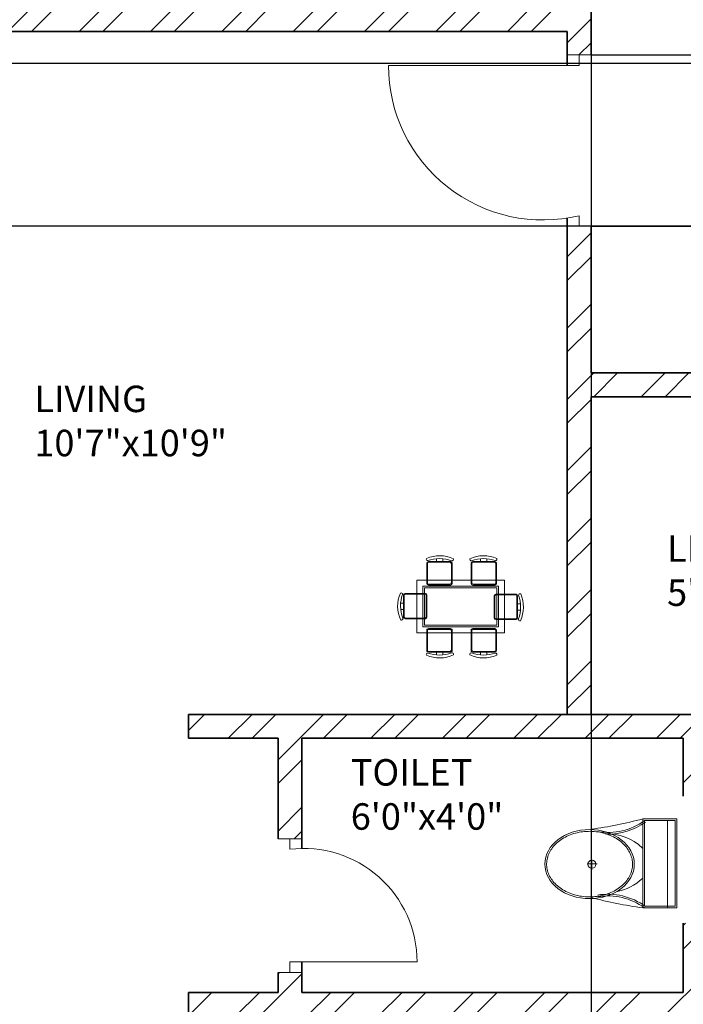
# Model space of a CAD drawing. Units: inches. Extents: x 1570 to 2186, y 1575 to 2421.
# Tile 3 of 10: x 1708 to 1833, y 1859 to 2045. Entities that reach past the tile are written whole.
import ezdxf

# ---------------------------------------------------------------- set-up
doc = ezdxf.new("R2010")
doc.units = ezdxf.units.IN
for name, color, linetype, lineweight in [('A-ANNO-DIMS', 2, 'Continuous', 18), ('A-AREA-IDEN', 7, 'Continuous', 18), ('A-DOOR', 201, 'Continuous', 18), ('A-FLOR-FIXT', 9, 'Continuous', 18), ('A-FURN', 8, 'Continuous', 13), ('A-WALL', 7, 'Continuous', 35), ('A-WALL-PATT', 252, 'Continuous', 13)]:
    doc.layers.add(name, color=color, linetype=linetype, lineweight=lineweight)
doc.styles.get("Standard").update_dxf_attribs({"font": 'arial.ttf'})
doc.dimstyles.get("Standard").update_dxf_attribs({"dimtxt": 0.18, "dimasz": 0.18, "dimexe": 0.18, "dimexo": 0.0625, "dimgap": 0.09, "dimtad": 0, "dimtih": 1, "dimtoh": 1, "dimdec": 4, "dimzin": 0, "dimdsep": 46, "dimtxsty": 'Standard', "dimcen": 0.09, "dimadec": 0, "dimazin": 0, "dimtfac": 1, "dimtdec": 4, "dimtofl": 0, "dimtmove": 0, "dimatfit": 3, "dimfxl": 1, "dimtolj": 1, "dimtzin": 0, "dimarcsym": 0})

# ---------------------------------------------------------------- blocks, each defined once
blk = doc.blocks.new('A$C31115884')
for p, q in [((257.5, 466.4), (257.5, 523.2)), ((283.1, 497.7), (223.4, 497.7)), ((0, 200), (0, 0)), ((520, 200), (0, 200)), ((10, 190), (10, 10)), ((510, 190), (10, 190)), ((510, 10), (510, 190)), ((520, 0), (520, 200)), ((510, 54.5), (0, 54.5)), ((10, 10), (510, 10)), ((0, 0), (520, 0))]:
    blk.add_line(p, q)
blk.add_circle((255.6, 496.4), 23.6)
for centre, radius, start, end in [((2777.7, -204.6), 2807, 165.4549, 171.71327), ((-294.5, 403.3), 364.7, 324.20913, 9.34987), ((-294.5, 403.3), 374.7, 324.20913, 9.34987), ((805.8, 403.3), 364.7, 170.65013, 215.79087), ((3237, 905), 2807, 188.28673, 194.5451), ((139.5, 406.2), 293.5, 315.84364, 2.65635), ((805.8, 403.3), 374.7, 179.20365, 215.79087), ((383.6, 406.2), 293.5, 190.27735, 224.15636)]:
    blk.add_arc(centre, radius, start, end)
blk.add_ellipse((256.2, 509.9), major_axis=(0, -260.7), ratio=0.772727)
blk.add_open_spline([(256.2, 259.2), (263.1, 259.2), (270, 259.7), (287.8, 262.3), (298.7, 265.1), (319.9, 273.1), (330.2, 278.4), (350.1, 291.1), (359.7, 298.7), (377.7, 315.9), (386.2, 325.5), (401.7, 346.6), (408.8, 358.1), (421.3, 382.5), (426.8, 395.5), (435.9, 422.4), (439.5, 436.4), (444.8, 465.1), (446.5, 479.7), (447.9, 509.2), (447.6, 524), (445, 553.3), (442.7, 567.8), (436.3, 596), (432.1, 609.7), (421.9, 636), (416, 648.6), (402.5, 672.1), (395, 683), (378.6, 703), (369.8, 712.1), (351.1, 728), (341.3, 734.8), (320.9, 746.2), (310.4, 750.7), (288.9, 757.3), (278, 759.4), (256, 761), (245, 760.6), (223.1, 757.2), (212.3, 754.3), (191.1, 746.1), (180.8, 740.7), (160.9, 727.8), (151.4, 720.1), (133.5, 702.7), (125.1, 693), (109.6, 671.7), (102.6, 660.2), (90.2, 635.7), (84.9, 622.7), (76, 595.6), (72.4, 581.6), (67.2, 552.9), (65.6, 538.2), (64.4, 508.8), (64.8, 494), (67.5, 464.7), (69.9, 450.2), (76.6, 422), (80.8, 408.3), (91.1, 382.2), (97.2, 369.7), (110.8, 346.3), (118.4, 335.4), (134.8, 315.6), (143.7, 306.7), (162.4, 290.9), (172.3, 284.2), (192.8, 273), (203.3, 268.6), (224.8, 262.2), (235.8, 260.2), (249.9, 259.3), (253, 259.2), (256.2, 259.2)], degree=3, knots=[0, 0, 0, 0, 0.110105, 0.110105, 0.285049, 0.285049, 0.459994, 0.459994, 0.634938, 0.634938, 0.809882, 0.809882, 0.984827, 0.984827, 1.159771, 1.159771, 1.334715, 1.334715, 1.50966, 1.50966, 1.684604, 1.684604, 1.859549, 1.859549, 2.034493, 2.034493, 2.209437, 2.209437, 2.384382, 2.384382, 2.559326, 2.559326, 2.73427, 2.73427, 2.909215, 2.909215, 3.084159, 3.084159, 3.259103, 3.259103, 3.434048, 3.434048, 3.608992, 3.608992, 3.783936, 3.783936, 3.958881, 3.958881, 4.133825, 4.133825, 4.30877, 4.30877, 4.483714, 4.483714, 4.658658, 4.658658, 4.833603, 4.833603, 5.008547, 5.008547, 5.183491, 5.183491, 5.358436, 5.358436, 5.53338, 5.53338, 5.708324, 5.708324, 5.883269, 5.883269, 6.058213, 6.058213, 6.233158, 6.233158, 6.283185, 6.283185, 6.283185, 6.283185])
blk = doc.blocks.new('TABLE-DINING')
for points in [[(0, 9.93), (16.54, 9.93), (16.54, 0), (0, 0)], [(0, 9.93), (16.54, 9.93), (16.54, 0), (0, 0)], [(1.1, 8.82), (15.44, 8.82), (15.44, 1.1), (1.1, 1.1)], [(1.1, 8.82), (15.44, 8.82), (15.44, 1.1), (1.1, 1.1)], [(1.43, 8.49), (15.11, 8.49), (15.11, 1.43), (1.43, 1.43)], [(1.43, 8.49), (15.11, 8.49), (15.11, 1.43), (1.43, 1.43)]]:
    blk.add_lwpolyline(points, close=True)
blk = doc.blocks.new('DINING-CHAIR-LH')
for points in [[(4.59, 1.1), (0.4, 1.1, -0.414214), (0.11, 1.39), (0.11, 5.24, -0.414214), (0.4, 5.53), (4.59, 5.53, -0.414214), (4.88, 5.24), (4.88, 1.39, -0.414214), (4.59, 1.1)], [(4.59, 1.1), (0.4, 1.1, -0.414214), (0.11, 1.39), (0.11, 5.24, -0.414214), (0.4, 5.53), (4.59, 5.53, -0.414214), (4.88, 5.24), (4.88, 1.39, -0.414214), (4.59, 1.1)], [(4.78, 0.96, -0.578392), (5.12, 0.58, -0.214524), (0.03, 0.51, -0.552014), (0.27, 0.92, 0.175809), (4.78, 0.96)], [(4.78, 0.96, -0.578392), (5.12, 0.58, -0.214524), (0.03, 0.51, -0.552014), (0.27, 0.92, 0.175809), (4.78, 0.96)], [(3.12, 1.1), (3.12, 0.57, 0.064759)], [(3.12, 1.1), (3.12, 0.57, 0.064759)]]:
    blk.add_lwpolyline(points, format="xyb")
blk.add_lwpolyline([(0.4, 1.23), (4.45, 1.23, 0.414214), (4.75, 1.53), (4.75, 5.11, 0.414214), (4.45, 5.4), (0.4, 5.4, 0.512069), (0.24, 5.11), (0.24, 1.53, 0.512069)], format="xyb", close=True)
blk.add_lwpolyline([(0.4, 1.23), (4.45, 1.23, 0.414214), (4.75, 1.53), (4.75, 5.11, 0.414214), (4.45, 5.4), (0.4, 5.4, 0.512069), (0.24, 5.11), (0.24, 1.53, 0.512069)], format="xyb", close=True)
blk.add_lwpolyline([(1.95, 0.56), (1.95, 1.1)])
blk.add_lwpolyline([(1.95, 0.56), (1.95, 1.1)])
blk = doc.blocks.new('DINING-CHAIR-RH')
for points in [[(4.73, 1.1, 0.414214), (5.02, 1.39), (5.02, 5.24, 0.414214), (4.73, 5.53), (0.55, 5.53, 0.414214), (0.25, 5.24), (0.25, 1.39, 0.414214), (0.55, 1.1), (4.73, 1.1)], [(4.73, 1.1, 0.414214), (5.02, 1.39), (5.02, 5.24, 0.414214), (4.73, 5.53), (0.55, 5.53, 0.414214), (0.25, 5.24), (0.25, 1.39, 0.414214), (0.55, 1.1), (4.73, 1.1)], [(4.86, 0.92, -0.175809), (0.35, 0.96, 0.578392), (0.01, 0.58, 0.214524), (5.1, 0.51, 0.552014), (4.86, 0.92, -0.065079)], [(4.86, 0.92, -0.175809), (0.35, 0.96, 0.578392), (0.01, 0.58, 0.214524), (5.1, 0.51, 0.552014), (4.86, 0.92, -0.065079)], [(2.02, 1.1), (2.02, 0.57, -0.064759)], [(2.02, 1.1), (2.02, 0.57, -0.064759)]]:
    blk.add_lwpolyline(points, format="xyb")
blk.add_lwpolyline([(4.73, 1.23), (0.68, 1.23, -0.414214), (0.39, 1.53), (0.39, 5.11, -0.414214), (0.68, 5.4), (4.73, 5.4, -0.512069), (4.89, 5.11), (4.89, 1.53, -0.512069)], format="xyb", close=True)
blk.add_lwpolyline([(4.73, 1.23), (0.68, 1.23, -0.414214), (0.39, 1.53), (0.39, 5.11, -0.414214), (0.68, 5.4), (4.73, 5.4, -0.512069), (4.89, 5.11), (4.89, 1.53, -0.512069)], format="xyb", close=True)
blk.add_lwpolyline([(3.19, 0.56), (3.19, 1.1)])
blk.add_lwpolyline([(3.19, 0.56), (3.19, 1.1)])
blk = doc.blocks.new('*D39')
at = {"layer": 'A-ANNO-DIMS', "color": 0, "lineweight": -2, "transparency": 16777216}
for p, q in [((1816.09, 2097.8), (1816.09, 1616.73)), ((1913.59, 2097.8), (1913.59, 1616.73)), ((1816.27, 1616.91), (1864.51, 1616.91)), ((1913.41, 1616.91), (1865.16, 1616.91))]:
    blk.add_line(p, q, dxfattribs=at)
at = {"layer": 'A-ANNO-DIMS', "color": 0, "transparency": 16777216}
for points in [[(1816.27, 1616.94), (1816.27, 1616.88), (1816.09, 1616.91)], [(1913.41, 1616.94), (1913.41, 1616.88), (1913.59, 1616.91)]]:
    blk.add_solid(points, dxfattribs=at)
at = {"layer": 'Defpoints', "color": 0, "transparency": 16777216}
for p in [(1816.09, 2097.86), (1913.59, 2097.86), (1913.59, 1616.91)]:
    blk.add_point(p, dxfattribs=at)
at = {"layer": 'A-ANNO-DIMS', "color": 0, "transparency": 16777216, "insert": (1864.84, 1616.91), "char_height": 0.18, "attachment_point": 5}
blk.add_mtext('\\A1;97.5', dxfattribs=at)
blk = doc.blocks.new('*D41')
at = {"layer": 'A-ANNO-DIMS', "color": 0, "lineweight": -2, "transparency": 16777216}
for p, q in [((1816.15, 2038.3), (2126.57, 2038.3)), ((2126.39, 2038.12), (2126.39, 2022.3)), ((2126.39, 2006.11), (2126.39, 2021.93)), ((1816.15, 2005.93), (2126.57, 2005.93))]:
    blk.add_line(p, q, dxfattribs=at)
at = {"layer": 'A-ANNO-DIMS', "color": 0, "transparency": 16777216}
for points in [[(2126.36, 2038.12), (2126.42, 2038.12), (2126.39, 2038.3)], [(2126.36, 2006.11), (2126.42, 2006.11), (2126.39, 2005.93)]]:
    blk.add_solid(points, dxfattribs=at)
at = {"layer": 'Defpoints', "color": 0, "transparency": 16777216}
for p in [(1816.09, 2038.3), (2126.39, 2038.3), (1816.09, 2005.93)]:
    blk.add_point(p, dxfattribs=at)
at = {"layer": 'A-ANNO-DIMS', "color": 0, "transparency": 16777216, "insert": (2126.39, 2022.12), "char_height": 0.18, "attachment_point": 5}
blk.add_mtext('\\A1;32.365', dxfattribs=at)
blk = doc.blocks.new('*D43')
at = {"layer": 'A-ANNO-DIMS', "color": 0, "lineweight": -2, "transparency": 16777216}
for p, q in [((1913.53, 2036.69), (1603.11, 2036.69)), ((1603.29, 2036.51), (1603.29, 2021.49)), ((1603.29, 2006.11), (1603.29, 2021.13)), ((1913.53, 2005.93), (1603.11, 2005.93))]:
    blk.add_line(p, q, dxfattribs=at)
at = {"layer": 'A-ANNO-DIMS', "color": 0, "transparency": 16777216}
for points in [[(1603.26, 2036.51), (1603.32, 2036.51), (1603.29, 2036.69)], [(1603.26, 2006.11), (1603.32, 2006.11), (1603.29, 2005.93)]]:
    blk.add_solid(points, dxfattribs=at)
at = {"layer": 'Defpoints', "color": 0, "transparency": 16777216}
for p in [(1603.29, 2036.69), (1913.59, 2036.69), (1913.59, 2005.93)]:
    blk.add_point(p, dxfattribs=at)
at = {"layer": 'A-ANNO-DIMS', "color": 0, "transparency": 16777216, "insert": (1603.29, 2021.31), "char_height": 0.18, "attachment_point": 5}
blk.add_mtext('\\A1;30.753', dxfattribs=at)

msp = doc.modelspace()

# ---------------------------------------------------------------- hatches: boundary and pattern name
at = {"layer": 'A-WALL-PATT'}
h = msp.add_hatch(dxfattribs=at)
h.set_pattern_fill('ANSI32', color=256)
h.paths.add_polyline_path([(1762.0975, 2362.1492), (1757.5975, 2362.1492), (1757.5975, 2357.6492), (1709.1163, 2357.6492), (1709.1163, 2362.1492), (1704.6163, 2362.1492), (1704.6163, 2353.1492), (1740.0886, 2353.1492), (1740.0886, 2261.8115), (1744.5886, 2261.8115), (1744.5886, 2353.1492), (1762.0975, 2353.1492)])
h.paths.add_polyline_path([(1890.2592, 2362.1492), (1885.7592, 2362.1492), (1826.5975, 2362.1492), (1822.0975, 2362.1492), (1822.0975, 2353.1492), (1862.5886, 2353.1492), (1862.5886, 2227.1492), (1744.5886, 2227.1492), (1744.5886, 2229.5389), (1742.3386, 2229.5389), (1740.0886, 2229.5389), (1740.0886, 2222.6492), (1744.5886, 2222.6492), (1756.186, 2222.6492), (1756.186, 2216.3571), (1760.686, 2216.3571), (1760.686, 2222.6492), (1832.686, 2222.6492), (1832.686, 2212.5994), (1837.186, 2212.5994), (1837.186, 2222.6492), (1893.186, 2222.6492), (1893.186, 2212.5994), (1897.686, 2212.5994), (1897.686, 2222.6492), (1989.5886, 2222.6492), (1989.5886, 2227.1492), (1989.5886, 2232.6585), (1987.3386, 2232.6585), (1985.0886, 2232.6585), (1985.0886, 2227.1492), (1867.0886, 2227.1492), (1867.0886, 2353.1492), (1890.2592, 2353.1492)])
h.paths.add_polyline_path([(1644.0886, 2353.1492), (1668.6163, 2353.1492), (1668.6163, 2362.1492), (1664.1163, 2362.1492), (1664.1163, 2358.9932), (1664.1163, 2357.6492), (1639.5886, 2357.6492), (1639.5886, 2213.8746), (1644.0886, 2213.8746), (1644.0886, 2222.6492), (1692.0886, 2222.6492), (1692.0886, 2215.9343), (1696.5886, 2215.9343), (1696.5886, 2222.6492), (1696.5886, 2227.1492), (1644.0886, 2227.1492)])
h.paths.add_polyline_path([(2013.0435, 2362.1492), (2008.5435, 2362.1492), (2008.5435, 2357.6492), (1954.7592, 2357.6492), (1954.7592, 2362.1492), (1950.2592, 2362.1492), (1950.2592, 2353.1492), (1985.0886, 2353.1492), (1985.0886, 2260.8534), (1989.5886, 2260.8534), (1989.5886, 2353.1492), (2013.0435, 2353.1492)])
h.paths.add_polyline_path([(2090.0886, 2357.6492), (2053.5435, 2357.6492), (2053.5435, 2362.1492), (2049.0435, 2362.1492), (2049.0435, 2353.1492), (2085.5886, 2353.1492), (2085.5886, 2227.1492), (2033.0886, 2227.1492), (2033.0886, 2222.6492), (2033.0886, 2214.4464), (2037.5886, 2214.4464), (2037.5886, 2222.6492), (2085.5886, 2222.6492), (2085.5886, 2212.4409), (2090.0886, 2212.4409)])
h.paths.add_polyline_path([(2090.0886, 2188.4409), (2087.8386, 2188.4409), (2085.5886, 2188.4409), (2085.5886, 2180.6492), (2037.5886, 2180.6492), (2037.5886, 2196.7956), (2033.0886, 2196.7956), (2033.0886, 2176.1492), (2037.5886, 2176.1492), (2045.0886, 2176.1492), (2045.0886, 2169.8988), (2049.5886, 2169.8988), (2049.5886, 2176.1492), (2085.5886, 2176.1492), (2085.5886, 2167.785), (2090.0886, 2167.785)])
h.paths.add_polyline_path([(2049.5886, 2147.4502), (2047.3386, 2147.4502), (2045.0886, 2147.4502), (2045.0886, 2124.4703), (2049.5886, 2124.4703)])
h.paths.add_polyline_path([(2090.0886, 2047.1492), (2049.5886, 2047.1492), (2049.5886, 2064.4703), (2045.0886, 2064.4703), (2045.0886, 2047.1492), (1918.0886, 2047.1492), (1918.0886, 2051.2061), (1913.5886, 2051.2061), (1913.5886, 2047.1492), (1913.5886, 2036.6872), (1918.0886, 2036.6872), (1918.0886, 2042.7492), (2045.0886, 2042.7492), (2045.0886, 2027.0686), (2049.5886, 2027.0686), (2049.5886, 2042.7492), (2090.0886, 2042.7492)])
h.paths.add_polyline_path([(1918.0886, 2005.9338), (1915.8386, 2005.9338), (1913.5886, 2005.9338), (1913.5886, 1913.7492), (1918.0886, 1913.7492)])
h.paths.add_polyline_path([(2090.0886, 1913.7492), (2049.5886, 1913.7492), (2045.0886, 1913.7492), (2033.0886, 1913.7492), (2033.0886, 1909.2492), (2033.0886, 1900.9803), (2037.5886, 1900.9803), (2037.5886, 1909.2492), (2085.5886, 1909.2492), (2085.5886, 1861.2492), (2037.5886, 1861.2492), (2037.5886, 1880.0859), (2033.0886, 1880.0859), (2033.0886, 1856.7492), (2085.5886, 1856.7492), (2085.5886, 1730.7492), (2054.2483, 1730.7492), (2054.2483, 1721.7492), (2058.7483, 1721.7492), (2058.7483, 1726.2492), (2090.0886, 1726.2492)])
h.paths.add_polyline_path([(2049.5886, 1967.0686), (2045.0886, 1967.0686), (2045.0886, 1913.7492), (2049.5886, 1913.7492)])
h.paths.add_polyline_path([(1989.5886, 1824.1695), (1987.3386, 1824.1695), (1985.0886, 1824.1695), (1985.0886, 1730.7492), (1989.5886, 1730.7492)])
h.paths.add_polyline_path([(1989.5886, 1861.2492), (1974.9963, 1861.2492), (1974.9963, 1865.9306), (1972.7463, 1865.9306), (1970.4963, 1865.9306), (1970.4963, 1861.2492), (1898.4963, 1861.2492), (1898.4963, 1874.2999), (1893.9963, 1874.2999), (1893.9963, 1861.2492), (1890.5886, 1861.2492), (1837.9963, 1861.2492), (1837.9963, 1874.3159), (1833.4963, 1874.3159), (1833.4963, 1861.2492), (1761.4963, 1861.2492), (1761.4963, 1865.0209), (1759.2463, 1865.0209), (1756.9963, 1865.0209), (1756.9963, 1861.2492), (1740.0886, 1861.2492), (1740.0886, 1856.7492), (1740.0886, 1850.7206), (1744.5886, 1850.7206), (1744.5886, 1856.7492), (1985.0886, 1856.7492), (1985.0886, 1851.0804), (1989.5886, 1851.0804), (1989.5886, 1856.7492)])
h.paths.add_polyline_path([(1989.5886, 1913.7492), (1740.0886, 1913.7492), (1740.0886, 1909.2492), (1756.9963, 1909.2492), (1756.9963, 1890.279), (1761.4963, 1890.279), (1761.4963, 1909.2492), (1833.4963, 1909.2492), (1833.4963, 1898.3159), (1837.9963, 1898.3159), (1837.9963, 1909.2492), (1890.5886, 1909.2492), (1893.9963, 1909.2492), (1893.9963, 1898.2999), (1898.4963, 1898.2999), (1898.4963, 1909.2492), (1970.4963, 1909.2492), (1970.4963, 1886.9887), (1974.9963, 1886.9887), (1974.9963, 1909.2492), (1989.5886, 1909.2492)])
h.paths.add_polyline_path([(1893.7344, 1730.7492), (1867.0886, 1730.7492), (1867.0886, 1856.7492), (1862.5886, 1856.7492), (1862.5886, 1730.7492), (1824.0492, 1730.7492), (1824.0492, 1721.7492), (1893.7344, 1721.7492)])
h.paths.add_polyline_path([(2018.2483, 1730.7492), (1953.7344, 1730.7492), (1953.7344, 1721.7492), (1958.2344, 1721.7492), (1958.2344, 1726.2492), (2013.7483, 1726.2492), (2013.7483, 1721.7492), (2018.2483, 1721.7492)])
h.paths.add_polyline_path([(1768.5492, 1730.7492), (1764.0492, 1730.7492), (1744.5886, 1730.7492), (1744.5886, 1819.4364), (1742.3386, 1819.4364), (1740.0886, 1819.4364), (1740.0886, 1730.7492), (1697.3801, 1730.7492), (1697.3801, 1721.7492), (1701.8801, 1721.7492), (1701.8801, 1726.2492), (1764.0492, 1726.2492), (1764.0492, 1721.7492), (1768.5492, 1721.7492)])
h.paths.add_polyline_path([(1644.0886, 1856.7492), (1639.5886, 1856.7492), (1639.5886, 1726.2492), (1657.0315, 1726.2492), (1657.0315, 1721.7492), (1661.3801, 1721.7492), (1661.3801, 1730.7492), (1644.0886, 1730.7492)])
h.paths.add_polyline_path([(1696.5886, 1876.1809), (1692.0886, 1876.1809), (1692.0886, 1861.2492), (1684.5886, 1861.2492), (1644.0886, 1861.2492), (1644.0886, 1909.2492), (1692.0886, 1909.2492), (1692.0886, 1900.3394), (1696.5886, 1900.3394), (1696.5886, 1913.7492), (1684.5886, 1913.7492), (1684.5886, 1920.2115), (1682.3386, 1920.2115), (1680.0886, 1920.2115), (1680.0886, 1913.7492), (1639.5886, 1913.7492), (1639.5886, 1856.7492), (1684.5886, 1856.7492), (1692.0886, 1856.7492), (1696.5886, 1856.7492)])
h.paths.add_polyline_path([(1684.5886, 2042.7492), (1811.5886, 2042.7492), (1811.5886, 2038.2991), (1816.0886, 2038.2991), (1816.0886, 2042.7492), (1816.0886, 2052.5708), (1813.8386, 2052.5708), (1811.5886, 2052.5708), (1811.5886, 2047.1492), (1684.5886, 2047.1492), (1684.5886, 2064.4703), (1680.0886, 2064.4703), (1680.0886, 2047.1492), (1639.5886, 2047.1492), (1639.5886, 2042.7492), (1680.0886, 2042.7492), (1680.0886, 2024.0762), (1684.5886, 2024.0762)])
h.paths.add_polyline_path([(1684.5886, 1964.0762), (1680.0886, 1964.0762), (1680.0886, 1944.6145), (1684.5886, 1944.6145)])
h.paths.add_polyline_path([(1816.0886, 1973.7492), (1876.0886, 1973.7492), (1876.0886, 1959.17), (1880.5886, 1959.17), (1880.5886, 1973.7492), (1880.5886, 1978.2492), (1816.0886, 1978.2492), (1816.0886, 2005.9338), (1813.8386, 2005.9338), (1811.5886, 2005.9338), (1811.5886, 1913.7492), (1816.0886, 1913.7492)])
h.paths.add_polyline_path([(1837.186, 2180.6492), (1837.186, 2188.5994), (1834.936, 2188.5994), (1832.686, 2188.5994), (1832.686, 2180.6492), (1760.686, 2180.6492), (1760.686, 2197.4807), (1756.186, 2197.4807), (1756.186, 2180.6492), (1744.5886, 2180.6492), (1740.0886, 2180.6492), (1740.0886, 2176.1492), (1837.186, 2176.1492)])
h.paths.add_polyline_path([(1974.186, 2196.8744), (1971.936, 2196.8744), (1969.686, 2196.8744), (1969.686, 2180.6492), (1897.686, 2180.6492), (1897.686, 2188.5994), (1895.436, 2188.5994), (1893.186, 2188.5994), (1893.186, 2180.6492), (1893.186, 2176.1492), (1974.186, 2176.1492)])
h.paths.add_polyline_path([(1918.0886, 2176.1492), (1913.5886, 2176.1492), (1913.5886, 2081.3709), (1918.0886, 2081.3709)])
h.paths.add_polyline_path([(1816.0886, 2176.1492), (1811.5886, 2176.1492), (1811.5886, 2081.3709), (1816.0886, 2081.3709)])
h.paths.add_polyline_path([(1684.5886, 2150.4939), (1682.3386, 2150.4939), (1680.0886, 2150.4939), (1680.0886, 2124.4703), (1684.5886, 2124.4703)])
h.paths.add_polyline_path([(1696.5886, 2180.6492), (1696.5886, 2197.4701), (1692.0886, 2197.4701), (1692.0886, 2180.6492), (1644.0886, 2180.6492), (1644.0886, 2189.8746), (1641.8386, 2189.8746), (1639.5886, 2189.8746), (1639.5886, 2169.814), (1644.0886, 2169.814), (1644.0886, 2176.1492), (1680.0886, 2176.1492), (1680.0886, 2171.7002), (1684.5886, 2171.7002), (1684.5886, 2176.1492), (1696.5886, 2176.1492)])

# ---------------------------------------------------------------- linework, layer by layer
at = {"layer": 'A-DOOR'}
for p, q in [((1811.5886, 2038.2991), (1816.0886, 2038.2991)), ((1816.0886, 2038.2991), (1813.8386, 2038.2991)), ((1813.8386, 2038.2991), (1813.8386, 2036.2991)), ((1813.8386, 2036.2991), (1777.8386, 2036.2991)), ((1813.8386, 2005.9338), (1813.8386, 2007.9338)), ((1811.5886, 2005.9338), (1816.0886, 2005.9338)), ((1816.0886, 2005.9338), (1813.8386, 2005.9338)), ((1756.9963, 1890.279), (1761.4963, 1890.279)), ((1761.4963, 1890.279), (1759.2463, 1890.279)), ((1759.2463, 1890.279), (1759.2463, 1888.279)), ((1759.2463, 1865.0209), (1759.2463, 1867.0209)), ((1759.2463, 1867.0209), (1783.2463, 1867.0209)), ((1756.9963, 1865.0209), (1761.4963, 1865.0209)), ((1761.4963, 1865.0209), (1759.2463, 1865.0209))]:
    msp.add_line(p, q, dxfattribs=at)
for centre, radius, start, end in [((1807.0135, 2036.2991), 29.1748, 180, 283.529154), ((1761.8316, 1867.0209), 21.4147, 360, 96.933842)]:
    msp.add_arc(centre, radius, start, end, dxfattribs=at)
at = {"layer": 'A-FURN'}
for points in [[(1785.2506, 1942.7954, -0.17580919), (1789.7564, 1942.7613, 0.57839206), (1790.0978, 1943.1367, 0.21452438), (1785.0116, 1943.2049, 0.55201397), (1785.2506, 1942.7954, -0.06507904)], [(1785.2506, 1942.7953, -0.17580919), (1789.7564, 1942.7611, 0.57839206), (1790.0978, 1943.1365, 0.21452438), (1785.0116, 1943.2047, 0.55201397), (1785.2506, 1942.7953, -0.06507904)], [(1793.5497, 1942.7613, -0.57839206), (1793.2084, 1943.1367, -0.21452438), (1798.2945, 1943.2049, -0.55201397), (1798.0556, 1942.7954, 0.1758092), (1793.5497, 1942.7613)], [(1793.5497, 1942.7611, -0.57839206), (1793.2084, 1943.1365, -0.21452438), (1798.2945, 1943.2047, -0.55201397), (1798.0556, 1942.7953, 0.1758092), (1793.5497, 1942.7611)], [(1789.5652, 1942.6146), (1785.3822, 1942.6146, 0.41421356), (1785.0895, 1942.3219), (1785.0895, 1938.4757, 0.41421356), (1785.3822, 1938.1831), (1789.5652, 1938.1831, 0.41421356), (1789.8579, 1938.4757), (1789.8579, 1942.3219, 0.41421356), (1789.5652, 1942.6146)], [(1789.5653, 1942.6144), (1785.3822, 1942.6144, 0.41421356), (1785.0895, 1942.3218), (1785.0895, 1938.4755, 0.41421356), (1785.3822, 1938.1829), (1789.5653, 1938.1829, 0.41421356), (1789.8579, 1938.4755), (1789.8579, 1942.3218, 0.41421356), (1789.5653, 1942.6144)], [(1788.0959, 1942.6146), (1788.0959, 1943.1436, -0.06475861)], [(1788.096, 1942.6144), (1788.096, 1943.1434, -0.06475861)], [(1797.9239, 1942.6146, -0.41421356), (1798.2166, 1942.3219), (1798.2166, 1938.4757, -0.41421356), (1797.9239, 1938.1831), (1793.7409, 1938.1831, -0.41421356), (1793.4482, 1938.4757), (1793.4482, 1942.3219, -0.41421356), (1793.7409, 1942.6146), (1797.9239, 1942.6146)], [(1797.924, 1942.6144, -0.41421356), (1798.2166, 1942.3218), (1798.2166, 1938.4755, -0.41421356), (1797.924, 1938.1829), (1793.7409, 1938.1829, -0.41421356), (1793.4483, 1938.4755), (1793.4483, 1942.3218, -0.41421356), (1793.7409, 1942.6144), (1797.924, 1942.6144)], [(1795.2102, 1942.6146), (1795.2102, 1943.1436, 0.06475861)], [(1795.2102, 1942.6144), (1795.2102, 1943.1434, 0.06475861)], [(1780.5366, 1931.9146, -0.57839206), (1780.1613, 1931.5732, -0.21452438), (1780.093, 1936.6593, -0.55201397), (1780.5025, 1936.4204, 0.17580937), (1780.5366, 1931.9146)], [(1780.5366, 1931.9144, -0.57839206), (1780.1613, 1931.573, -0.21452438), (1780.093, 1936.6591, -0.55201397), (1780.5025, 1936.4202, 0.17580937), (1780.5366, 1931.9144)], [(1780.6833, 1936.2888, -0.41421356), (1780.976, 1936.5814), (1784.8222, 1936.5814, -0.41421356), (1785.1149, 1936.2888), (1785.1149, 1932.1057, -0.41421356), (1784.8222, 1931.8131), (1780.976, 1931.8131, -0.41421356), (1780.6833, 1932.1057), (1780.6833, 1936.2888)], [(1780.6834, 1936.2886, -0.41421356), (1780.976, 1936.5812), (1784.8222, 1936.5812, -0.41421356), (1785.1149, 1936.2886), (1785.1149, 1932.1055, -0.41421356), (1784.8222, 1931.8129), (1780.976, 1931.8129, -0.41421356), (1780.6834, 1932.1055), (1780.6834, 1936.2886)], [(1802.2241, 1936.1455, 0.41421356), (1801.9315, 1936.4382), (1798.0852, 1936.4382, 0.41421356), (1797.7926, 1936.1455), (1797.7926, 1931.9625, 0.41421356), (1798.0852, 1931.6698), (1801.9315, 1931.6698, 0.41421356), (1802.2241, 1931.9625), (1802.2241, 1936.1455)], [(1802.2241, 1936.1453, 0.41421356), (1801.9315, 1936.438), (1798.0852, 1936.438, 0.41421356), (1797.7926, 1936.1453), (1797.7926, 1931.9623, 0.41421356), (1798.0852, 1931.6696), (1801.9315, 1931.6696, 0.41421356), (1802.2241, 1931.9623), (1802.2241, 1936.1453)], [(1802.405, 1936.2771, -0.17580919), (1802.3708, 1931.7713, 0.57839206), (1802.7462, 1931.4299, 0.21452438), (1802.8144, 1936.5161, 0.55201397), (1802.405, 1936.2771, -0.06507904)], [(1802.405, 1936.2769, -0.17580919), (1802.3709, 1931.7711, 0.57839206), (1802.7462, 1931.4298, 0.21452438), (1802.8144, 1936.5159, 0.55201397), (1802.405, 1936.2769, -0.06507904)], [(1780.6833, 1933.575), (1780.1543, 1933.575, 0.06475861)], [(1780.6834, 1933.5748), (1780.1543, 1933.5748, 0.06475861)], [(1802.2241, 1933.4318), (1802.7532, 1933.4318, -0.06475861)], [(1802.2241, 1933.4316), (1802.7532, 1933.4316, -0.06475861)]]:
    msp.add_lwpolyline(points, format="xyb", dxfattribs=at)
for points in [[(1785.384, 1942.4828), (1789.4334, 1942.4828, -0.41421356), (1789.7261, 1942.1901), (1789.7261, 1938.6075, -0.41421356), (1789.4334, 1938.3149), (1785.384, 1938.3149, -0.51206948), (1785.2214, 1938.6075), (1785.2214, 1942.1901, -0.51206948)], [(1785.384, 1942.4826), (1789.4334, 1942.4826, -0.41421356), (1789.7261, 1942.1899), (1789.7261, 1938.6074, -0.41421356), (1789.4334, 1938.3147), (1785.384, 1938.3147, -0.51206948), (1785.2214, 1938.6074), (1785.2214, 1942.1899, -0.51206948)], [(1797.9222, 1942.4828), (1793.8727, 1942.4828, 0.41421356), (1793.5801, 1942.1901), (1793.5801, 1938.6075, 0.41421356), (1793.8727, 1938.3149), (1797.9222, 1938.3149, 0.51206948), (1798.0848, 1938.6075), (1798.0848, 1942.1901, 0.51206948)], [(1797.9222, 1942.4826), (1793.8727, 1942.4826, 0.41421356), (1793.5801, 1942.1899), (1793.5801, 1938.6074, 0.41421356), (1793.8727, 1938.3147), (1797.9222, 1938.3147, 0.51206948), (1798.0848, 1938.6074), (1798.0848, 1942.1899, 0.51206948)], [(1780.8152, 1936.287), (1780.8152, 1932.2376, 0.41421356), (1781.1078, 1931.9449), (1784.6904, 1931.9449, 0.41421356), (1784.983, 1932.2376), (1784.983, 1936.287, 0.51206948), (1784.6904, 1936.4496), (1781.1078, 1936.4496, 0.51206948)], [(1780.8152, 1936.2868), (1780.8152, 1932.2374, 0.41421356), (1781.1078, 1931.9447), (1784.6904, 1931.9447, 0.41421356), (1784.9831, 1932.2374), (1784.9831, 1936.2868, 0.51206948), (1784.6904, 1936.4494), (1781.1078, 1936.4494, 0.51206948)], [(1802.0923, 1936.1437), (1802.0923, 1932.0943, -0.41421356), (1801.7996, 1931.8016), (1798.2171, 1931.8016, -0.41421356), (1797.9244, 1932.0943), (1797.9244, 1936.1437, -0.51206948), (1798.2171, 1936.3063), (1801.7996, 1936.3063, -0.51206948)], [(1802.0923, 1936.1436), (1802.0923, 1932.0941, -0.41421356), (1801.7996, 1931.8015), (1798.2171, 1931.8015, -0.41421356), (1797.9244, 1932.0941), (1797.9244, 1936.1436, -0.51206948), (1798.2171, 1936.3061), (1801.7996, 1936.3061, -0.51206948)]]:
    msp.add_lwpolyline(points, format="xyb", close=True, dxfattribs=at)
for points in [[(1786.925, 1943.1532), (1786.925, 1942.6146)], [(1786.9251, 1943.1531), (1786.9251, 1942.6144)], [(1796.3811, 1943.1532), (1796.3811, 1942.6146)], [(1796.3811, 1943.1531), (1796.3811, 1942.6144)], [(1780.1447, 1934.7459), (1780.6833, 1934.7459)], [(1780.1447, 1934.7457), (1780.6834, 1934.7457)], [(1802.7628, 1934.6027), (1802.2241, 1934.6027)], [(1802.7628, 1934.6025), (1802.2241, 1934.6025)]]:
    msp.add_lwpolyline(points, dxfattribs=at)
at = {"layer": 'A-WALL'}
for p, q in [((1816.0886, 2052.5708), (1816.0886, 2042.7492)), ((1684.5886, 2042.7492), (1811.5886, 2042.7492)), ((1811.5886, 2042.7492), (1684.5886, 2042.7492)), ((1811.5886, 2042.7492), (1811.5886, 2036.2991)), ((1816.0886, 2038.2991), (1816.0886, 2042.7492)), ((1811.5886, 2007.4852), (1811.5886, 1913.7492)), ((1816.0886, 1978.2492), (1816.0886, 2005.9338)), ((1880.5886, 1978.2492), (1816.0886, 1978.2492)), ((1816.0886, 1913.7492), (1816.0886, 1973.7492)), ((1816.0886, 1913.7492), (1816.0886, 1973.7492)), ((1816.0886, 1973.7492), (1876.0886, 1973.7492)), ((1740.0886, 1913.7492), (1740.0886, 1909.2492)), ((1989.5886, 1913.7492), (1740.0886, 1913.7492)), ((1811.5886, 1913.7492), (1816.0886, 1913.7492)), ((1756.9963, 1909.2492), (1740.0886, 1909.2492)), ((1756.9963, 1890.279), (1756.9963, 1909.2492)), ((1833.4963, 1909.2492), (1761.4963, 1909.2492)), ((1761.4963, 1909.2492), (1761.4963, 1888.433)), ((1833.4963, 1909.2492), (1761.4963, 1909.2492)), ((1833.4963, 1909.2492), (1830.0886, 1909.2492)), ((1833.4963, 1909.2492), (1833.4963, 1898.3159)), ((1833.4963, 1874.3159), (1833.4963, 1861.2492)), ((1761.4963, 1867.0209), (1761.4963, 1861.2492)), ((1756.9963, 1861.2492), (1756.9963, 1865.0209)), ((1740.0886, 1861.2492), (1740.0886, 1856.7492)), ((1756.9963, 1861.2492), (1740.0886, 1861.2492)), ((1833.4963, 1861.2492), (1761.4963, 1861.2492))]:
    msp.add_line(p, q, dxfattribs=at)

# ---------------------------------------------------------------- block references
at = {"layer": 'A-FLOR-FIXT', "xscale": 0.0323450304620732, "yscale": 0.0323450304620732, "zscale": 0.0323450304620732, "rotation": 89.99999999999996}
msp.add_blockref('A$C31115884', (1832.3007, 1877.1919), dxfattribs=at)
at = {"layer": 'A-FURN'}
for name, p in [('TABLE-DINING', (1783.204, 1929.156)), ('DINING-CHAIR-LH', (1784.98, 1924.415)), ('DINING-CHAIR-RH', (1793.195, 1924.415))]:
    msp.add_blockref(name, p, dxfattribs=at)

# ---------------------------------------------------------------- texts
at = {"layer": 'A-AREA-IDEN', "char_height": 5, "attachment_point": 1}
for s, width, insert in [('LIVING\\P10\'7"x10\'9"', 173.320071, (1710.9984, 1975.8372)), ('LIFT\\P5\'0"x5\'0"', 119.411331, (1830.4398, 1947.5705)), ('TOILET\\P6\'0"x4\'0"', 95.131267, (1770.727, 1905.3043))]:
    msp.add_mtext_dynamic_manual_height_columns(s, width=width, gutter_width=12.5, heights=[0], dxfattribs=dict(at, insert=insert))

# ---------------------------------------------------------------- dimensions: what is measured, and where the dimension line sits
at = {"layer": 'A-ANNO-DIMS'}
dim = msp.add_linear_dim(base=(1913.5886, 1616.9104), p1=(1816.0886, 2097.8597), p2=(1913.5886, 2097.8597), dimstyle='Standard', override={"dimdec": 1, "dimlfac": 1, "dimrnd": 0, "dimzin": 0, "dimdsep": 46, "dimlunit": 2}, dxfattribs=at)
dim.commit()
dim.dimension.update_dxf_attribs({"geometry": '*D39', "text_midpoint": (1864.8386, 1616.9104)})
for base, p1, p2, picture, middle in [((2126.3886, 2038.2991), (1816.0886, 2005.9338), (1816.0886, 2038.2991), '*D41', (2126.3886, 2022.1164)), ((1603.2886, 2036.6872), (1913.5886, 2005.9338), (1913.5886, 2036.6872), '*D43', (1603.2886, 2021.3105))]:
    dim = msp.add_linear_dim(base=base, p1=p1, p2=p2, angle=90, dimstyle='Standard', override={"dimdec": 3, "dimlfac": 1, "dimrnd": 0, "dimzin": 0, "dimdsep": 46, "dimlunit": 2}, dxfattribs=at)
    dim.commit()
    dim.dimension.update_dxf_attribs({"geometry": picture, "text_midpoint": middle})

doc.saveas('drawing.dxf')
